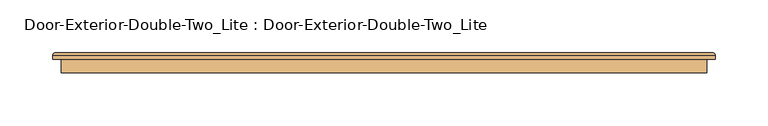
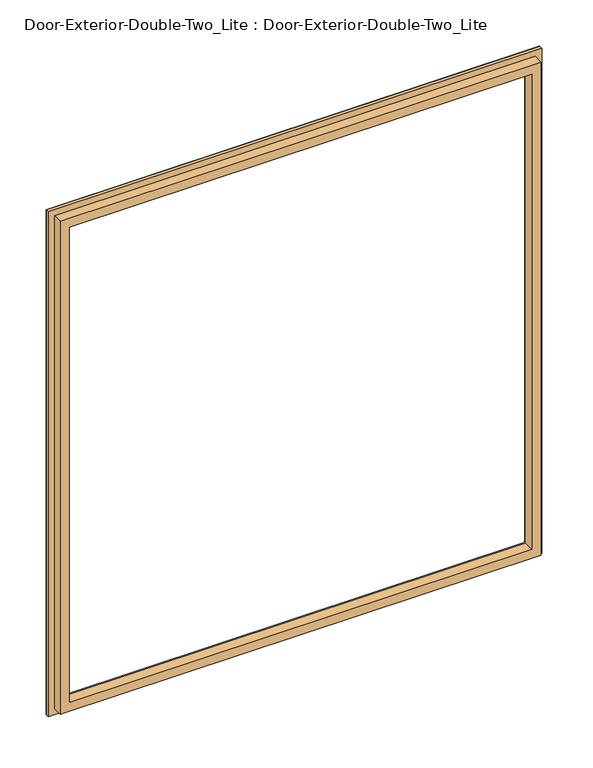
"""IFC4 building model written with IfcOpenShell, lengths in millimetres: door geometry, Door-Exterior-Double-Two_Lite : Door-Exterior-Double-Two_Lite."""

from ifc_helpers import new_model, si_unit, frame, origin, place, context, project, spatial, ellipse_curve, source, transform, mapped, element, save
from ifc_brep_helpers import plane_surface, cylinder_surface, advanced_brep


def door_exterior_double_two_lite_door_exterior_double_two_lite_037690dd(model_context):
    return source(origin(), model_context, "Body", "AdvancedBrep", [
        advanced_brep(
        [(-762.0, 118.25, 914.4), (-762.0, 130.95, 914.4), (-762.0, 130.95, 254.0), (-762.0, 118.25, 254.0), (-750.0, 131.95, 902.4), (-750.0, 118.25, 902.4), (-750.0, 118.25, 266.0), (-750.0, 131.95, 266.0), (-755.0, 136.95, 907.4), (-755.0, 136.95, 261.0), (-770.0, 134.95, 922.4), (-768.0, 136.95, 920.4), (-768.0, 136.95, 248.0), (-770.0, 134.95, 246.0), (-770.0, 130.95, 922.4), (-770.0, 130.95, 246.0), (-152.4, 130.95, 254.0), (-152.4, 118.25, 254.0), (-164.4, 118.25, 266.0), (-164.4, 131.95, 266.0), (-159.4, 136.95, 261.0), (-146.4, 136.95, 248.0), (-144.4, 134.95, 246.0), (-144.4, 130.95, 246.0), (-152.4, 130.95, 914.4), (-152.4, 118.25, 914.4), (-164.4, 118.25, 902.4), (-164.4, 131.95, 902.4), (-159.4, 136.95, 907.4), (-146.4, 136.95, 920.4), (-144.4, 134.95, 922.4), (-144.4, 130.95, 922.4)],
        [
            (0, 1),
            (1, 2),
            (2, 3),
            (3, 0),
            (4, 5),
            (5, 6),
            (6, 7),
            (7, 4),
            (8, 4, ellipse_curve(frame((-755.0, 131.95, 907.4), z_axis=(-0.7071067811865475, 0.0, -0.7071067811865475), x_axis=(-0.7071067811865474, 0.0, 0.7071067811865476)), 7.0710678, 5.0)),
            (7, 9, ellipse_curve(frame((-755.0, 131.95, 261.0), z_axis=(-0.7071067811865475, 0.0, 0.7071067811865475), x_axis=(0.7071067811865474, 0.0, 0.7071067811865476)), 7.0710678, 5.0)),
            (9, 8),
            (10, 11, ellipse_curve(frame((-768.0, 134.95, 920.4), z_axis=(-0.7071067811865475, 0.0, -0.7071067811865475), x_axis=(-0.7071067811865474, 0.0, 0.7071067811865476)), 2.8284271, 2.0)),
            (11, 12),
            (12, 13, ellipse_curve(frame((-768.0, 134.95, 248.0), z_axis=(-0.7071067811865475, 0.0, 0.7071067811865475), x_axis=(0.7071067811865474, 0.0, 0.7071067811865476)), 2.8284271, 2.0)),
            (13, 10),
            (14, 10),
            (13, 15),
            (15, 14),
            (2, 16),
            (16, 17),
            (17, 3),
            (6, 18),
            (18, 19),
            (19, 7),
            (19, 20, ellipse_curve(frame((-159.4, 131.95, 261.0), z_axis=(-0.7071067811865475, 0.0, -0.7071067811865475), x_axis=(-0.7071067811865476, 0.0, 0.7071067811865474)), 7.0710678, 5.0)),
            (20, 9),
            (12, 21),
            (21, 22, ellipse_curve(frame((-146.4, 134.95, 248.0), z_axis=(-0.7071067811865475, 0.0, -0.7071067811865475), x_axis=(-0.7071067811865476, 0.0, 0.7071067811865474)), 2.8284271, 2.0)),
            (22, 13),
            (22, 23),
            (23, 15),
            (16, 24),
            (24, 25),
            (25, 17),
            (18, 26),
            (26, 27),
            (27, 19),
            (27, 28, ellipse_curve(frame((-159.4, 131.95, 907.4), z_axis=(0.7071067811865475, 0.0, -0.7071067811865475), x_axis=(-0.7071067811865474, 0.0, -0.7071067811865476)), 7.0710678, 5.0)),
            (28, 20),
            (21, 29),
            (29, 30, ellipse_curve(frame((-146.4, 134.95, 920.4), z_axis=(0.7071067811865475, 0.0, -0.7071067811865475), x_axis=(-0.7071067811865474, 0.0, -0.7071067811865476)), 2.8284271, 2.0)),
            (30, 22),
            (30, 31),
            (31, 23),
            (31, 14),
            (1, 24),
            (0, 25),
            (5, 26),
            (4, 27),
            (8, 28),
            (11, 29),
            (10, 30),
        ],
        [
            plane_surface(frame((-762.0, 130.95, 914.4), z_axis=(-1.0, 0.0, 0.0), x_axis=(0.0, 0.0, -1.0))),
            plane_surface(frame((-750.0, 118.25, 902.4), z_axis=(1.0, 0.0, 0.0), x_axis=(0.0, 0.0, -1.0))),
            cylinder_surface(frame((-755.0, 131.95, 914.4), z_axis=(0.0, 0.0, 1.0), x_axis=(-1.0, 0.0, 0.0)), 5.0),
            cylinder_surface(frame((-768.0, 134.95, 914.4), z_axis=(0.0, 0.0, 1.0), x_axis=(-1.0, 0.0, 0.0)), 2.0),
            plane_surface(frame((-770.0, 134.95, 922.4), z_axis=(-1.0, 0.0, 0.0), x_axis=(0.0, 0.0, -1.0))),
            plane_surface(frame((-762.0, 130.95, 254.0), z_axis=(0.0, 0.0, -1.0), x_axis=(1.0, 0.0, 0.0))),
            plane_surface(frame((-750.0, 118.25, 266.0), z_axis=(0.0, 0.0, 1.0), x_axis=(1.0, 0.0, 0.0))),
            cylinder_surface(frame((-762.0, 131.95, 261.0), z_axis=(-1.0, 0.0, 0.0), x_axis=(0.0, 0.0, -1.0)), 5.0),
            cylinder_surface(frame((-762.0, 134.95, 248.0), z_axis=(-1.0, 0.0, 0.0), x_axis=(0.0, 0.0, -1.0)), 2.0),
            plane_surface(frame((-770.0, 134.95, 246.0), z_axis=(0.0, 0.0, -1.0), x_axis=(1.0, 0.0, 0.0))),
            plane_surface(frame((-152.4, 130.95, 254.0), z_axis=(1.0, 0.0, 0.0), x_axis=(0.0, 0.0, 1.0))),
            plane_surface(frame((-164.4, 118.25, 266.0), z_axis=(-1.0, 0.0, 0.0), x_axis=(0.0, 0.0, 1.0))),
            cylinder_surface(frame((-159.4, 131.95, 254.0), z_axis=(0.0, 0.0, -1.0), x_axis=(1.0, 0.0, 0.0)), 5.0),
            cylinder_surface(frame((-146.4, 134.95, 254.0), z_axis=(0.0, 0.0, -1.0), x_axis=(1.0, 0.0, 0.0)), 2.0),
            plane_surface(frame((-144.4, 134.95, 246.0), z_axis=(1.0, 0.0, 0.0), x_axis=(0.0, 0.0, 1.0))),
            plane_surface(frame((-144.4, 130.95, 922.4), z_axis=(0.0, -1.0, 0.0), x_axis=(-1.0, 0.0, 0.0))),
            plane_surface(frame((-152.4, 130.95, 914.4), z_axis=(0.0, 0.0, 1.0), x_axis=(-1.0, 0.0, 0.0))),
            plane_surface(frame((-152.4, 118.25, 914.4), z_axis=(0.0, -1.0, 0.0), x_axis=(-1.0, 0.0, 0.0))),
            plane_surface(frame((-164.4, 118.25, 902.4), z_axis=(0.0, 0.0, -1.0), x_axis=(-1.0, 0.0, 0.0))),
            cylinder_surface(frame((-152.4, 131.95, 907.4), z_axis=(1.0, 0.0, 0.0), x_axis=(0.0, 0.0, 1.0)), 5.0),
            plane_surface(frame((-159.4, 136.95, 907.4), z_axis=(0.0, 1.0, 0.0), x_axis=(-1.0, 0.0, 0.0))),
            cylinder_surface(frame((-152.4, 134.95, 920.4), z_axis=(1.0, 0.0, 0.0), x_axis=(0.0, 0.0, 1.0)), 2.0),
            plane_surface(frame((-144.4, 134.95, 922.4), z_axis=(0.0, 0.0, 1.0), x_axis=(-1.0, 0.0, 0.0))),
        ],
        [
            (0, [[1, 2, 3, 4]]),
            (1, [[5, 6, 7, 8]]),
            (2, [[9, -8, 10, 11]]),
            (3, [[12, 13, 14, 15]]),
            (4, [[16, -15, 17, 18]]),
            (5, [[-3, 19, 20, 21]]),
            (6, [[-7, 22, 23, 24]]),
            (7, [[-10, -24, 25, 26]]),
            (8, [[-14, 27, 28, 29]]),
            (9, [[-17, -29, 30, 31]]),
            (10, [[-20, 32, 33, 34]]),
            (11, [[-23, 35, 36, 37]]),
            (12, [[-25, -37, 38, 39]]),
            (13, [[-28, 40, 41, 42]]),
            (14, [[-30, -42, 43, 44]]),
            (15, [[-31, -44, 45, -18], [46, -32, -19, -2]]),
            (16, [[-33, -46, -1, 47]]),
            (17, [[-21, -34, -47, -4], [48, -35, -22, -6]]),
            (18, [[-36, -48, -5, 49]]),
            (19, [[-38, -49, -9, 50]]),
            (20, [[51, -40, -27, -13], [-26, -39, -50, -11]]),
            (21, [[-41, -51, -12, 52]]),
            (22, [[-43, -52, -16, -45]]),
        ],
    ),
    ])


if __name__ == "__main__":
    model = new_model("IFC4")
    model_context = context("Model", 3, world=origin())
    ifc_project = project(units=[si_unit("LENGTHUNIT", "METRE", prefix="MILLI")], contexts=[model_context])
    site = spatial("IfcSite", under=ifc_project)
    building = spatial("IfcBuilding", under=site)
    placement = place(None, origin())
    door_exterior_double_two_lite_door_exterior_double_two_lite_shape = door_exterior_double_two_lite_door_exterior_double_two_lite_037690dd(model_context)
    element("IfcDoor", 1, ObjectType="Door-Exterior-Double-Two_Lite : Door-Exterior-Double-Two_Lite", at=placement, inside=building, context=model_context, shape_type="MappedRepresentation", body=[
        mapped(door_exterior_double_two_lite_door_exterior_double_two_lite_shape, transform((0.0, 0.0, 0.0), x_axis=(1.0, 0.0, 0.0), y_axis=(0.0, 1.0, 0.0), z_axis=(0.0, 0.0, 1.0))),
    ])
    save(model, "model.ifc")

# Revit data of these elements
# Type "Door-Exterior-Double-Two_Lite : Door-Exterior-Double-Two_Lite"
#   Type Mark = "48"
#   Assembly Code = "B2030100"
#   Analytic Construction = "Metal frame, double glass door"
#   Top Rail = 117.475 mm
#   Threshold Length [instance default] = 1930.4 mm
#   Threshold Offset [instance default] = 12.7 mm
#   Thickness = 44.45 mm
#   Thermal Resistance (R) = 0.242926 (m²·K)/W
#   Swing Angle [instance default] = 90.00°
#   Strike Height = 1016 mm
#   Stiles = 152.4 mm
#   SinglePanelWidth = 914.4 mm
#   Rough Width [instance default] = 1930.4 mm
#   Rough Height [instance default] = 2235.2 mm
#   MFOpeningHeight [instance default] = 101.6 mm
#   MFOpeningWidth [instance default] = 101.6 mm
#   Lock Rail = 203.2 mm
#   Inset Calculate [instance default] = 101.6 mm
#   Masonry Inset [instance default] = 25.4 mm
#   Height = 2133.6 mm
#   Width = 1828.8 mm
#   Heat Transfer Coefficient (U) = 4.11674 W/(m²·K)
#   Glass Thickness = 19.05 mm
#   Masonry Frame Depth = 146.05 mm
#   Bottom Rail = 254 mm
#   Threshold [instance default] = yes
#   Masonry Frame [instance default] = yes
#   Function = 1
#   Dry Wall Frame [instance default] = no
#   Threshold Material = none
#   Panic Bar Material = Metal - Stainless Steel
#   Panel Material = Metal - Painted - Grey
#   Glass Stop Material = Metal - Painted - Grey
#   Frame Material = Metal - Painted - Grey
#   Exterior Pull Material = Metal - Stainless Steel
#   Visual Light Transmittance = 0
#   Solar Heat Gain Coefficient = 0
#   Wall Closure = (empty or 0)
# Element 1 (IfcDoor, "Door-Exterior-Double-Two_Lite : Door-Exterior-Double-Two_Lite")
#   Materials on its faces: "Metal - Painted - Grey", "Metal - Stainless Steel", "Glass", "Door - Frame/Mullion"
# Materials
#   "Metal - Stainless Steel": class "Metal", colour RGB 247 247 247, transparency 0
#   "Metal - Painted - Grey": class "Paint", colour RGB 104 104 104, transparency 0
#   "Glass": class "Glass", colour RGB 0 128 192, transparency 0.9, Description = "Soda Lime Glass", Cost = 0
#   "Door - Frame/Mullion": class "Wood", colour RGB 212 179 113, transparency 0, Keynote = "L20", Cost = 0
